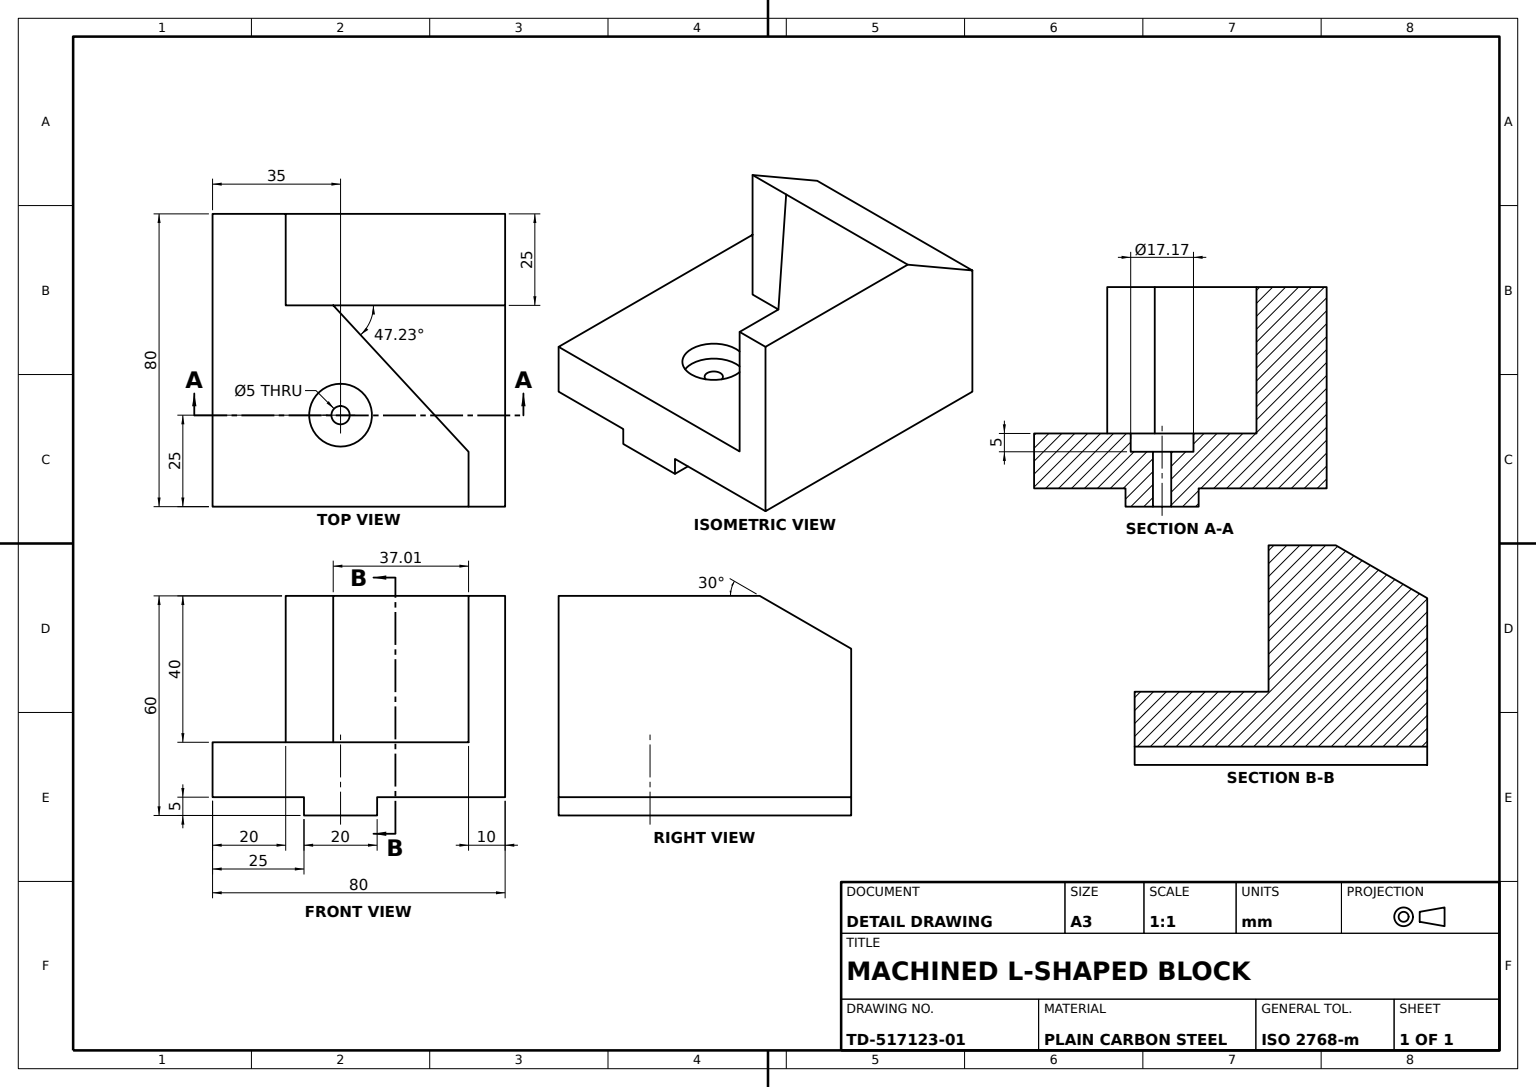
from build123d import *

# Parameters (mm, degrees)
BASE_PROFILE_SKETCH_W       = 80
BASE_PROFILE_SKETCH_H       = 20
BASE_BLOCK_DEPTH            = 80
UNDERSIDE_SLOT_SKETCH_W     = 25
UNDERSIDE_SLOT_SKETCH_H     = 5
UNDERSIDE_SLOT_SKETCH_W_2   = 35
UNDERSIDE_SLOT_DEPTH        = 80
UPRIGHT_WALL_SKETCH_W       = 10
UPRIGHT_WALL_SKETCH_H       = 80
UPRIGHT_WALL_DEPTH          = 40
SIDE_BLOCK_DEPTH            = 40
WALL_CHAMFER_25X30DEG_SIZE  = 25
WALL_CHAMFER_25X30DEG_SIZE2 = 14.43375673
COUNTERBORE_SKETCH_R        = 8.583879332
COUNTERBORE_RECESS_DEPTH    = 5
HOLE_SKETCH_R               = 2.5
HOLE_DIA5_DEPTH             = 22


with BuildPart() as part:
    # Base Profile Sketch → Base Block (new body)
    with BuildSketch(Plane.XY):
        Rectangle(BASE_PROFILE_SKETCH_W, BASE_PROFILE_SKETCH_H)
    extrude(amount=BASE_BLOCK_DEPTH)

    # Underside Slot Sketch → Underside Slot (cut)
    with BuildSketch(Plane.XY.offset(80)):
        with Locations((-27.5, -7.5)):
            Rectangle(UNDERSIDE_SLOT_SKETCH_W, UNDERSIDE_SLOT_SKETCH_H)
        with Locations((22.5, -7.5)):
            Rectangle(UNDERSIDE_SLOT_SKETCH_W_2, UNDERSIDE_SLOT_SKETCH_H)
    extrude(amount=-UNDERSIDE_SLOT_DEPTH, mode=Mode.SUBTRACT)

    # Upright Wall Sketch → Upright Wall (add)
    with BuildSketch(Plane(origin=(0, 10, 0), x_dir=(1, 0, 0), z_dir=(0, 1, 0))):
        with Locations((35, -40)):
            Rectangle(UPRIGHT_WALL_SKETCH_W, UPRIGHT_WALL_SKETCH_H)
    extrude(amount=UPRIGHT_WALL_DEPTH)

    # Side Block Sketch → Side Block (add)
    with BuildSketch(Plane(origin=(0, 10, 0), x_dir=(1, 0, 0), z_dir=(0, 1, 0))):
        Polygon((-20, 0), (-20, -25), (-7.006583052, -25), (30, -65), (30, 0), align=None)
    extrude(amount=SIDE_BLOCK_DEPTH)

    # Wall Chamfer 25x30deg
    wall_chamfer_25x30deg_edges = [part.edges().sort_by_distance(p)[0] for p in [
        (10, 50, 0),
    ]]
    wall_chamfer_25x30deg_side = [part.faces().sort_by_distance(p)[0] for p in [
        (16.961219392, 50, 27.237680119),
    ]]
    chamfer(wall_chamfer_25x30deg_edges, length=WALL_CHAMFER_25X30DEG_SIZE, length2=WALL_CHAMFER_25X30DEG_SIZE2, reference=wall_chamfer_25x30deg_side[0])

    # Counterbore Sketch → Counterbore Recess (cut)
    with BuildSketch(Plane(origin=(0, 10, 0), x_dir=(1, 0, 0), z_dir=(0, 1, 0))):
        with Locations(Location((-5, -55, 0), (0, 0, 270))):
            Circle(COUNTERBORE_SKETCH_R)
    extrude(amount=-COUNTERBORE_RECESS_DEPTH, mode=Mode.SUBTRACT)

    # Hole Sketch → Hole Dia5 (cut)
    with BuildSketch(Plane(origin=(0, 5, 0), x_dir=(1, 0, 0), z_dir=(0, 1, 0))):
        with Locations(Location((-5, -55, 0), (0, 0, 270))):
            Circle(HOLE_SKETCH_R)
    extrude(amount=-HOLE_DIA5_DEPTH, mode=Mode.SUBTRACT)


solid = part.part
